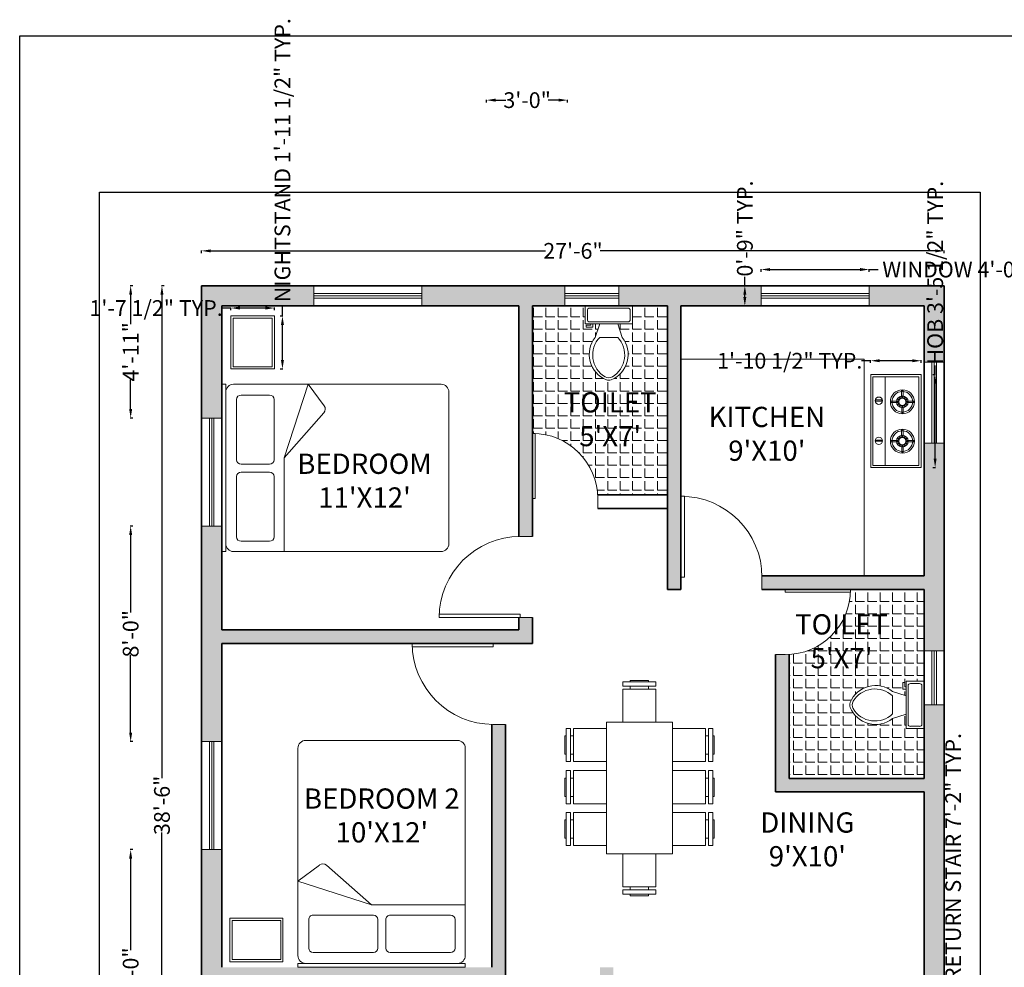
# Model space of a CAD drawing. Units: inches. Extents: x -80 to 1461, y -1239 to 153.
# Tile 3 of 6: x -80 to 358, y -273 to 149. Entities that reach past the tile are written whole.
import ezdxf

# ---------------------------------------------------------------- set-up
doc = ezdxf.new("R2010")
doc.units = ezdxf.units.IN
doc.header["$MEASUREMENT"] = 0
for name, color, linetype, lineweight in [('A-ANNO-DIMS', 2, 'Continuous', 18), ('A-ANNO-TTLB', 7, 'Continuous', 25), ('A-AREA-IDEN', 7, 'Continuous', 18), ('A-EQPM', 8, 'Continuous', 18), ('A-FLOR-FIXT', 9, 'Continuous', 18), ('A-FLOR-PATT', 143, 'Continuous', 13), ('A-FURN', 8, 'Continuous', 18), ('A-GLAZ', 4, 'Continuous', 18), ('A-WALL', 7, 'Continuous', 35), ('A-WALL-PATT', 8, 'Continuous', 13), ('DOOR', 32, 'Continuous', 18)]:
    doc.layers.add(name, color=color, linetype=linetype, lineweight=lineweight)
doc.styles.get("Standard").update_dxf_attribs({"font": 'arial.ttf'})
doc.dimstyles.get("Standard").update_dxf_attribs({"dimtxt": 7, "dimasz": 4, "dimexe": 0.18, "dimexo": 0.0625, "dimgap": 0.09, "dimtad": 0, "dimdec": 0, "dimzin": 0, "dimdsep": 46, "dimlunit": 3, "dimtxsty": 'Standard', "dimcen": 0.09, "dimadec": 0, "dimazin": 0, "dimtfac": 1, "dimtdec": 0, "dimtofl": 0, "dimtmove": 0, "dimatfit": 3, "dimfxl": 1, "dimfxlon": 1, "dimtolj": 1, "dimtzin": 0, "dimarcsym": 0})

# ---------------------------------------------------------------- blocks, each defined once
blk = doc.blocks.new('*U2')
for p, q in [((0, 0), (0, -6)), ((40, 0), (40, -6))]:
    blk.add_line(p, q)
blk.add_lwpolyline([(0, 0), (0, 40), (1.75, 40), (1.75, 0)], close=True)
blk.add_arc((0, 0), 40, 0, 90)
blk = doc.blocks.new('A$C164346CA')
for p, q in [((0, 2.035), (0, 2)), ((1.5, 2.035), (0, 2.035)), ((1.5, 2), (1.5, 2.035)), ((1.5, 2), (0, 2)), ((0, 1.93), (0, 0.07)), ((0.0919, 1.8624), (0.0919, 1.6069)), ((0.6731, 1.9024), (0.1319, 1.9024)), ((0.7131, 1.6069), (0.7131, 1.8624)), ((0.7828, 1.8624), (0.7828, 1.6069)), ((1.364, 1.9024), (0.8228, 1.9024)), ((1.404, 1.6069), (1.404, 1.8624)), ((1.5, 0.07), (1.5, 1.93)), ((0.1319, 1.5669), (0.6731, 1.5669)), ((0.8228, 1.5669), (1.364, 1.5669)), ((0.8395, 1.4761), (0, 1.4761)), ((0.8395, 1.4761), (1.2448, 1.12)), ((1.5, 1.2611), (0.8395, 1.4761)), ((1.3077, 1.1175), (1.5, 1.2611)), ((0.07, 0), (1.43, 0))]:
    blk.add_line(p, q)
for centre, radius, start, end in [((0.07, 1.93), 0.07, 90, 180), ((1.43, 1.93), 0.07, 0, 90), ((0.1319, 1.8624), 0.04, 90, 180), ((0.6731, 1.8624), 0.04, 0, 90), ((0.8228, 1.8624), 0.04, 90, 180), ((1.364, 1.8624), 0.04, 0, 90), ((0.1319, 1.6069), 0.04, 180, 270), ((0.6731, 1.6069), 0.04, 270, 0), ((0.8228, 1.6069), 0.04, 180, 270), ((1.364, 1.6069), 0.04, 270, 0), ((1.2778, 1.1575), 0.05, 228.69584, 306.75789), ((0.07, 0.07), 0.07, 180, 270), ((1.43, 0.07), 0.07, 270, 0)]:
    blk.add_arc(centre, radius, start, end)
blk = doc.blocks.new('*U5')
for p, q in [((241, -152), (241, -51)), ((-254, -216), (-203, -216)), ((-254, -241), (-254, -216)), ((-203, -216), (-203, -203)), ((-178, -203), (-178, -241)), ((-102, -203), (-152, -356)), ((102, -203), (152, -356)), ((-178, -241), (-254, -241)), ((102, -356), (-102, -356))]:
    blk.add_line(p, q)
blk.add_lwpolyline([(267, -203), (267, 0), (-267, 0), (-267, -203)], close=True)
for points in [[(-241, -51), (-241, -152)], [(216, -25), (-216, -25)], [(-216, -178), (216, -178)]]:
    blk.add_lwpolyline(points)
for centre, radius, start, end in [((-219, -48), 22.5, 81.8699, 188.1301), ((219, -48), 22.5, 351.8699, 98.1301), ((-219, -156), 22.5, 171.8699, 278.1301), ((219, -156), 22.5, 261.8699, 8.1301), ((89, -548), 309, 141.4691, 247.9714), ((107, -554), 288, 136.3677, 238.9468), ((-89, -548), 309, 292.0284, 38.5307), ((-107, -554), 288, 301.053, 43.6321), ((0, -708), 102, 245.7318, 294.2682), ((0, -737), 102, 254.8605, 285.1395)]:
    blk.add_arc(centre, radius, start, end)
blk = doc.blocks.new('A$C06E242FC')
for p, q in [((0, 455.6), (0.5, 456.1)), ((0, 455.6), (0, 0.5)), ((838.9, 456.1), (0.5, 456.1)), ((838.9, 456.1), (839.4, 455.6)), ((839.4, 0.5), (839.4, 455.6)), ((20, 435.6), (20.5, 436.1)), ((20, 435.6), (20, 20.5)), ((818.9, 436.1), (20.5, 436.1)), ((237.3, 411.5), (237.3, 356.2)), ((248.9, 411.5), (237.3, 411.5)), ((237.3, 356.2), (248.9, 356.2)), ((248.9, 356.2), (248.9, 411.5)), ((599.3, 411.5), (610.9, 411.5)), ((599.3, 411.5), (599.3, 356.2)), ((599.3, 356.2), (610.9, 356.2)), ((610.9, 356.2), (610.9, 411.5)), ((819.4, 435.6), (818.9, 436.1)), ((819.4, 20.5), (819.4, 435.6)), ((20, 324.4), (819.4, 324.4)), ((232.7, 272.7), (232.7, 214)), ((244.9, 272.7), (232.7, 272.7)), ((244.9, 214), (244.9, 272.7)), ((588.1, 272.7), (588.1, 214)), ((600.3, 272.7), (588.1, 272.7)), ((600.3, 214), (600.3, 272.7)), ((232.7, 214), (244.9, 214)), ((588.1, 214), (600.3, 214)), ((136.3, 176), (136.3, 163.8)), ((194.9, 176), (136.3, 176)), ((136.3, 163.8), (194.9, 163.8)), ((194.9, 163.8), (194.9, 176)), ((245.2, 126.1), (233, 126.1)), ((233, 126.1), (233, 67.4)), ((245.2, 67.4), (245.2, 126.1)), ((282.9, 176.3), (282.9, 164.1)), ((341.6, 176.3), (282.9, 176.3)), ((282.9, 164.1), (341.6, 164.1)), ((341.6, 164.1), (341.6, 176.3)), ((550.3, 176), (491.7, 176)), ((491.7, 176), (491.7, 163.8)), ((491.7, 163.8), (550.3, 163.8)), ((550.3, 163.8), (550.3, 176)), ((600.6, 126.1), (588.3, 126.1)), ((588.3, 126.1), (588.3, 67.4)), ((600.6, 67.4), (600.6, 126.1)), ((638.3, 176.3), (638.3, 164.1)), ((697, 176.3), (638.3, 176.3)), ((638.3, 164.1), (697, 164.1)), ((697, 164.1), (697, 176.3)), ((0, 0.5), (0.5, 0)), ((20, 20.5), (20.5, 20)), ((20.5, 20), (818.9, 20)), ((233, 67.4), (245.2, 67.4)), ((588.3, 67.4), (600.6, 67.4)), ((818.9, 20), (819.4, 20.5)), ((838.9, 0), (839.4, 0.5)), ((0.5, 0), (838.9, 0))]:
    blk.add_line(p, q)
for centre, radius in [((242, 382.9), 33.3), ((604.1, 382.9), 33.3), ((238.9, 170.1), 108.3), ((594.3, 170.1), 108.3), ((238.9, 170.1), 93.3), ((238.9, 170.1), 52.6), ((205.3, 189.5), 4.84), ((238.9, 170.1), 32.6), ((219.5, 203.7), 4.84), ((238.9, 208.9), 4.84), ((258.4, 203.7), 4.84), ((272.6, 189.5), 4.84), ((594.3, 170.1), 93.3), ((594.3, 170.1), 52.6), ((560.7, 189.5), 4.84), ((594.3, 170.1), 32.6), ((574.9, 203.7), 4.84), ((594.3, 208.9), 4.84), ((613.7, 203.7), 4.84), ((628, 189.5), 4.84), ((200.1, 170.1), 4.84), ((205.3, 150.6), 4.84), ((219.5, 136.4), 4.84), ((238.9, 131.2), 4.84), ((258.4, 136.4), 4.84), ((272.6, 150.6), 4.84), ((277.8, 170.1), 4.84), ((555.5, 170.1), 4.84), ((560.7, 150.6), 4.84), ((574.9, 136.4), 4.84), ((594.3, 131.2), 4.84), ((613.7, 136.4), 4.84), ((628, 150.6), 4.84), ((633.2, 170.1), 4.84)]:
    blk.add_circle(centre, radius)
blk = doc.blocks.new('A$C4C0603CD')
for p, q in [((1.106, 2.02), (0.656, 2.02)), ((0.656, 2.02), (0.656, 1.96)), ((1.006, 2.04), (0.756, 2.04)), ((0.756, 2.04), (0.756, 2.02)), ((1.006, 2.02), (1.006, 2.04)), ((1.106, 1.96), (1.106, 2.02)), ((1.232, 2.02), (1.232, 1.96)), ((1.684, 2.02), (1.232, 2.02)), ((1.584, 2.04), (1.334, 2.04)), ((1.334, 2.04), (1.334, 2.02)), ((1.584, 2.02), (1.584, 2.04)), ((1.684, 1.96), (1.684, 2.02)), ((1.802, 2.02), (1.802, 1.96)), ((2.252, 2.02), (1.802, 2.02)), ((2.152, 2.04), (1.902, 2.04)), ((1.902, 2.04), (1.902, 2.02)), ((2.152, 2.02), (2.152, 2.04)), ((2.252, 1.96), (2.252, 2.02)), ((1.106, 1.96), (0.656, 1.96)), ((0.656, 1.92), (0.656, 1.47)), ((1.106, 1.92), (0.656, 1.92)), ((0.756, 1.96), (0.756, 1.92)), ((1.006, 1.92), (1.006, 1.96)), ((1.106, 1.47), (1.106, 1.92)), ((1.684, 1.96), (1.232, 1.96)), ((1.232, 1.92), (1.232, 1.47)), ((1.684, 1.92), (1.232, 1.92)), ((1.334, 1.96), (1.334, 1.92)), ((1.584, 1.92), (1.584, 1.96)), ((1.684, 1.47), (1.684, 1.92)), ((2.252, 1.96), (1.802, 1.96)), ((1.802, 1.92), (1.802, 1.47)), ((2.252, 1.92), (1.802, 1.92)), ((1.902, 1.96), (1.902, 1.92)), ((2.152, 1.92), (2.152, 1.96)), ((2.252, 1.47), (2.252, 1.92)), ((0.57, 1.47), (0.57, 0.57)), ((2.37, 1.47), (0.57, 1.47)), ((0.656, 1.47), (1.106, 1.47)), ((1.107, 1.47), (1.684, 1.47)), ((1.802, 1.47), (2.252, 1.47)), ((2.37, 1.47), (2.37, 0.57)), ((0.02, 1.245), (0.02, 0.795)), ((0.08, 1.245), (0.02, 1.245)), ((0.08, 1.245), (0.08, 0.795)), ((0.12, 1.245), (0.12, 0.795)), ((0.57, 1.245), (0.12, 1.245)), ((0.57, 0.795), (0.57, 1.245)), ((2.37, 1.245), (2.37, 0.795)), ((2.82, 1.245), (2.37, 1.245)), ((2.82, 0.795), (2.82, 1.245)), ((2.86, 0.795), (2.86, 1.245)), ((2.92, 1.245), (2.86, 1.245)), ((2.92, 0.795), (2.92, 1.245)), ((0, 1.145), (0, 0.895)), ((0.02, 1.145), (0, 1.145)), ((0.12, 1.145), (0.08, 1.145)), ((2.86, 1.145), (2.82, 1.145)), ((2.94, 1.145), (2.92, 1.145)), ((2.94, 0.895), (2.94, 1.145)), ((0, 0.895), (0.02, 0.895)), ((0.08, 0.895), (0.12, 0.895)), ((2.82, 0.895), (2.86, 0.895)), ((2.92, 0.895), (2.94, 0.895)), ((0.02, 0.795), (0.08, 0.795)), ((0.12, 0.795), (0.57, 0.795)), ((2.37, 0.795), (2.82, 0.795)), ((2.86, 0.795), (2.92, 0.795)), ((0.57, 0.57), (2.37, 0.57)), ((1.106, 0.57), (0.656, 0.57)), ((0.656, 0.57), (0.656, 0.12)), ((1.106, 0.12), (1.106, 0.57)), ((1.684, 0.57), (1.232, 0.57)), ((1.232, 0.57), (1.232, 0.12)), ((1.684, 0.12), (1.684, 0.57)), ((2.252, 0.57), (1.802, 0.57)), ((1.802, 0.57), (1.802, 0.12)), ((2.252, 0.12), (2.252, 0.57)), ((0.656, 0.12), (1.106, 0.12)), ((0.656, 0.08), (1.106, 0.08)), ((0.656, 0.08), (0.656, 0.02)), ((0.656, 0.02), (1.106, 0.02)), ((0.756, 0.12), (0.756, 0.08)), ((0.756, 0.02), (0.756, 0)), ((0.756, 0), (1.006, 0)), ((1.006, 0.08), (1.006, 0.12)), ((1.006, 0), (1.006, 0.02)), ((1.106, 0.02), (1.106, 0.08)), ((1.232, 0.12), (1.684, 0.12)), ((1.232, 0.08), (1.684, 0.08)), ((1.232, 0.08), (1.232, 0.02)), ((1.232, 0.02), (1.684, 0.02)), ((1.334, 0.12), (1.334, 0.08)), ((1.334, 0.02), (1.334, 0)), ((1.334, 0), (1.584, 0)), ((1.584, 0.08), (1.584, 0.12)), ((1.584, 0), (1.584, 0.02)), ((1.684, 0.02), (1.684, 0.08)), ((1.802, 0.12), (2.252, 0.12)), ((1.802, 0.08), (2.252, 0.08)), ((1.802, 0.08), (1.802, 0.02)), ((1.802, 0.02), (2.252, 0.02)), ((1.902, 0.12), (1.902, 0.08)), ((1.902, 0.02), (1.902, 0)), ((1.902, 0), (2.152, 0)), ((2.152, 0.08), (2.152, 0.12)), ((2.152, 0), (2.152, 0.02)), ((2.252, 0.02), (2.252, 0.08))]:
    blk.add_line(p, q)
blk = doc.blocks.new('*D11')
at = {"layer": 'A-ANNO-DIMS', "color": 0, "lineweight": -2, "transparency": 16777216}
for p, q in [((0.99, 44.81), (0.99, 45.99)), ((4.99, 45.81), (153.82, 45.81)), ((326.99, 45.81), (178.16, 45.81)), ((330.99, 44.81), (330.99, 45.99))]:
    blk.add_line(p, q, dxfattribs=at)
at = {"layer": 'A-ANNO-DIMS', "color": 0, "transparency": 16777216}
for points in [[(4.99, 46.47), (4.99, 45.14), (0.99, 45.81)], [(326.99, 46.47), (326.99, 45.14), (330.99, 45.81)]]:
    blk.add_solid(points, dxfattribs=at)
at = {"layer": 'Defpoints', "color": 0, "transparency": 16777216}
for p in [(330.99, 45.81), (0.99, 30.32), (330.99, 30.32)]:
    blk.add_point(p, dxfattribs=at)
at = {"layer": 'A-ANNO-DIMS', "color": 0, "transparency": 16777216, "insert": (165.99, 45.81), "char_height": 7, "attachment_point": 5}
blk.add_mtext('\\A1;27\'-6"', dxfattribs=at)
blk = doc.blocks.new('*D12')
at = {"layer": 'A-ANNO-DIMS', "color": 0, "lineweight": -2, "transparency": 16777216}
for p, q in [((-15.61, 30.32), (-16.79, 30.32)), ((-16.61, 26.32), (-16.61, -188.57)), ((-16.61, -427.68), (-16.61, -212.8)), ((-15.61, -431.68), (-16.79, -431.68))]:
    blk.add_line(p, q, dxfattribs=at)
at = {"layer": 'A-ANNO-DIMS', "color": 0, "transparency": 16777216}
for points in [[(-17.27, 26.32), (-15.94, 26.32), (-16.61, 30.32)], [(-17.27, -427.68), (-15.94, -427.68), (-16.61, -431.68)]]:
    blk.add_solid(points, dxfattribs=at)
at = {"layer": 'Defpoints', "color": 0, "transparency": 16777216}
for p in [(0.99, 30.32), (-16.61, -431.68), (0.99, -431.68)]:
    blk.add_point(p, dxfattribs=at)
at = {"layer": 'A-ANNO-DIMS', "color": 0, "transparency": 16777216, "insert": (-16.61, -200.68), "char_height": 7, "attachment_point": 5, "rotation": 90}
blk.add_mtext('\\A1;38\'-6"', dxfattribs=at)
blk = doc.blocks.new('WIN-48IN')
for p, q in [((0, 9), (0, 0)), ((48, 9), (0, 9)), ((48, 0), (48, 9)), ((0, 5.5), (48, 5.5)), ((0, 4.5), (48, 4.5)), ((0, 3.5), (48, 3.5)), ((0, 0), (36, 0)), ((36, 0), (48, 0))]:
    blk.add_line(p, q)
blk = doc.blocks.new('WIN-24IN')
for p, q in [((0, 9), (0, 0)), ((0, 9), (24, 9)), ((24, 9), (24, 0)), ((0, 5.5), (24, 5.5)), ((0, 4.5), (24, 4.5)), ((0, 3.5), (24, 3.5)), ((0, 0), (24, 0))]:
    blk.add_line(p, q)
blk = doc.blocks.new('WIN-36IN')
for p, q in [((0, 36), (9, 36)), ((0, 36), (0, 0)), ((3.5, 0), (3.5, 36)), ((4.5, 0), (4.5, 36)), ((5.5, 0), (5.5, 36)), ((9, 0), (9, 36)), ((0, 0), (9, 0))]:
    blk.add_line(p, q)
blk = doc.blocks.new('NIGHTSTAND')
for points in [[(0, 19.36), (23.56, 19.36), (23.56, 0), (0, 0)], [(1, 18.36), (22.56, 18.36), (22.56, 1), (1, 1)]]:
    blk.add_lwpolyline(points, close=True)
blk = doc.blocks.new('COUNTER-L-PLAN')
for p, q in [((0, 96.29), (81.45, 96.29)), ((81.45, 96.29), (81.45, 0))]:
    blk.add_line(p, q)
blk = doc.blocks.new('*D36')
at = {"layer": 'A-ANNO-DIMS', "color": 0, "lineweight": -2, "transparency": 16777216}
for p, q in [((249.57, 36.52), (249.57, 37.7)), ((253.57, 37.52), (293.57, 37.52)), ((297.57, 36.52), (297.57, 37.7)), ((297.57, 37.52), (301.57, 37.52))]:
    blk.add_line(p, q, dxfattribs=at)
at = {"layer": 'A-ANNO-DIMS', "color": 0, "transparency": 16777216}
for points in [[(253.57, 38.18), (253.57, 36.85), (249.57, 37.52)], [(293.57, 38.18), (293.57, 36.85), (297.57, 37.52)]]:
    blk.add_solid(points, dxfattribs=at)
at = {"layer": 'Defpoints', "color": 0, "transparency": 16777216}
for p in [(297.57, 37.52), (249.57, 30.32), (297.57, 30.32)]:
    blk.add_point(p, dxfattribs=at)
at = {"layer": 'A-ANNO-DIMS', "color": 0, "transparency": 16777216, "insert": (345.95, 37.52), "char_height": 7, "attachment_point": 5}
blk.add_mtext('\\A1;WINDOW 4\'-0" TYP.', dxfattribs=at)
blk = doc.blocks.new('*D37')
at = {"layer": 'A-ANNO-DIMS', "color": 0, "lineweight": -2, "transparency": 16777216}
for p, q in [((242.37, 30.32), (242.37, 34.32)), ((243.37, 30.32), (242.19, 30.32)), ((242.37, 25.32), (242.37, 26.32)), ((243.37, 21.32), (242.19, 21.32))]:
    blk.add_line(p, q, dxfattribs=at)
at = {"layer": 'A-ANNO-DIMS', "color": 0, "transparency": 16777216}
for points in [[(241.7, 26.32), (243.03, 26.32), (242.37, 30.32)], [(241.7, 25.32), (243.03, 25.32), (242.37, 21.32)]]:
    blk.add_solid(points, dxfattribs=at)
at = {"layer": 'Defpoints', "color": 0, "transparency": 16777216}
for p in [(242.37, 30.32), (249.57, 30.32), (249.57, 21.32)]:
    blk.add_point(p, dxfattribs=at)
at = {"layer": 'A-ANNO-DIMS', "color": 0, "transparency": 16777216, "insert": (242.37, 55.74), "char_height": 7, "attachment_point": 5, "rotation": 90}
blk.add_mtext('\\A1;0\'-9" TYP.', dxfattribs=at)
blk = doc.blocks.new('*D48')
at = {"layer": 'A-ANNO-DIMS', "color": 0, "lineweight": -2, "transparency": 16777216}
for p, q in [((36.92, 16.87), (36.92, 20.87)), ((35.92, 16.87), (37.1, 16.87)), ((36.92, -2.69), (36.92, 12.87)), ((35.92, -6.69), (37.1, -6.69))]:
    blk.add_line(p, q, dxfattribs=at)
at = {"layer": 'A-ANNO-DIMS', "color": 0, "transparency": 16777216}
for points in [[(36.25, 12.87), (37.59, 12.87), (36.92, 16.87)], [(36.25, -2.69), (37.59, -2.69), (36.92, -6.69)]]:
    blk.add_solid(points, dxfattribs=at)
at = {"layer": 'Defpoints', "color": 0, "transparency": 16777216}
for p in [(33.39, 16.87), (36.92, 16.87), (33.39, -6.69)]:
    blk.add_point(p, dxfattribs=at)
at = {"layer": 'A-ANNO-DIMS', "color": 0, "transparency": 16777216, "insert": (36.92, 86.13), "char_height": 7, "attachment_point": 5, "rotation": 90}
blk.add_mtext('\\A1;NIGHTSTAND 1\'-11 1/2" TYP.', dxfattribs=at)
blk = doc.blocks.new('*D49')
at = {"layer": 'A-ANNO-DIMS', "color": 0, "lineweight": -2, "transparency": 16777216}
for p, q in [((14.03, 20.4), (10.03, 20.4)), ((14.03, 19.4), (14.03, 20.58)), ((29.39, 20.4), (18.03, 20.4)), ((33.39, 19.4), (33.39, 20.58))]:
    blk.add_line(p, q, dxfattribs=at)
at = {"layer": 'A-ANNO-DIMS', "color": 0, "transparency": 16777216}
for points in [[(18.03, 21.07), (18.03, 19.73), (14.03, 20.4)], [(29.39, 21.07), (29.39, 19.73), (33.39, 20.4)]]:
    blk.add_solid(points, dxfattribs=at)
at = {"layer": 'Defpoints', "color": 0, "transparency": 16777216}
for p in [(14.03, 20.4), (14.03, 16.87), (33.39, 16.87)]:
    blk.add_point(p, dxfattribs=at)
at = {"layer": 'A-ANNO-DIMS', "color": 0, "transparency": 16777216, "insert": (-19.22, 20.4), "char_height": 7, "attachment_point": 5}
blk.add_mtext('\\A1;1\'-7 1/2" TYP.', dxfattribs=at)
blk = doc.blocks.new('*D50')
at = {"layer": 'A-ANNO-DIMS', "color": 0, "lineweight": -2, "transparency": 16777216}
for p, q in [((326.92, -9.22), (326.92, -5.22)), ((325.92, -9.22), (327.1, -9.22)), ((326.92, -46.53), (326.92, -13.22)), ((325.92, -50.53), (327.1, -50.53))]:
    blk.add_line(p, q, dxfattribs=at)
at = {"layer": 'A-ANNO-DIMS', "color": 0, "transparency": 16777216}
for points in [[(326.25, -13.22), (327.58, -13.22), (326.92, -9.22)], [(326.25, -46.53), (327.58, -46.53), (326.92, -50.53)]]:
    blk.add_solid(points, dxfattribs=at)
at = {"layer": 'Defpoints', "color": 0, "transparency": 16777216}
for p in [(320.72, -9.22), (326.92, -9.22), (320.72, -50.53)]:
    blk.add_point(p, dxfattribs=at)
at = {"layer": 'A-ANNO-DIMS', "color": 0, "transparency": 16777216, "insert": (326.92, 36.12), "char_height": 7, "attachment_point": 5, "rotation": 90}
blk.add_mtext('\\A1;HOB 3\'-5 1/2" TYP.', dxfattribs=at)
blk = doc.blocks.new('*D51')
at = {"layer": 'A-ANNO-DIMS', "color": 0, "lineweight": -2, "transparency": 16777216}
for p, q in [((298.27, -3.03), (294.27, -3.03)), ((298.27, -4.03), (298.27, -2.85)), ((316.72, -3.03), (302.27, -3.03)), ((320.72, -4.03), (320.72, -2.85))]:
    blk.add_line(p, q, dxfattribs=at)
at = {"layer": 'A-ANNO-DIMS', "color": 0, "transparency": 16777216}
for points in [[(302.27, -2.36), (302.27, -3.69), (298.27, -3.03)], [(316.72, -2.36), (316.72, -3.69), (320.72, -3.03)]]:
    blk.add_solid(points, dxfattribs=at)
at = {"layer": 'Defpoints', "color": 0, "transparency": 16777216}
for p in [(298.27, -3.03), (298.27, -9.22), (320.72, -9.22)]:
    blk.add_point(p, dxfattribs=at)
at = {"layer": 'A-ANNO-DIMS', "color": 0, "transparency": 16777216, "insert": (262.3, -3.03), "char_height": 7, "attachment_point": 5}
blk.add_mtext('\\A1;1\'-10 1/2" TYP.', dxfattribs=at)
blk = doc.blocks.new('*D56')
at = {"layer": 'A-ANNO-DIMS', "color": 0, "lineweight": -2, "transparency": 16777216}
for p, q in [((334.89, -286.42), (334.89, -282.42)), ((333.89, -286.42), (335.07, -286.42)), ((334.89, -368.42), (334.89, -290.42)), ((333.89, -372.42), (335.07, -372.42))]:
    blk.add_line(p, q, dxfattribs=at)
at = {"layer": 'A-ANNO-DIMS', "color": 0, "transparency": 16777216}
for points in [[(334.22, -290.42), (335.56, -290.42), (334.89, -286.42)], [(334.22, -368.42), (335.56, -368.42), (334.89, -372.42)]]:
    blk.add_solid(points, dxfattribs=at)
at = {"layer": 'Defpoints', "color": 0, "transparency": 16777216}
for p in [(321.99, -286.42), (334.89, -286.42), (321.99, -372.42)]:
    blk.add_point(p, dxfattribs=at)
at = {"layer": 'A-ANNO-DIMS', "color": 0, "transparency": 16777216, "insert": (334.89, -223.69), "char_height": 7, "attachment_point": 5, "rotation": 90}
blk.add_mtext('\\A1;RETURN STAIR 7\'-2" TYP.', dxfattribs=at)
blk = doc.blocks.new('*D72')
at = {"layer": 'A-ANNO-DIMS', "color": 0, "lineweight": -2, "transparency": 16777216}
for p, q in [((412.49, 30.32), (413.67, 30.32)), ((413.49, 26.32), (413.49, -224.38)), ((413.49, -499.58), (413.49, -248.89)), ((412.49, -503.58), (413.67, -503.58))]:
    blk.add_line(p, q, dxfattribs=at)
at = {"layer": 'A-ANNO-DIMS', "color": 0, "transparency": 16777216}
for points in [[(412.82, 26.32), (414.16, 26.32), (413.49, 30.32)], [(412.82, -499.58), (414.16, -499.58), (413.49, -503.58)]]:
    blk.add_solid(points, dxfattribs=at)
at = {"layer": 'Defpoints', "color": 0, "transparency": 16777216}
for p in [(330.99, 30.32), (183.99, -503.58), (413.49, -503.58)]:
    blk.add_point(p, dxfattribs=at)
at = {"layer": 'A-ANNO-DIMS', "color": 0, "transparency": 16777216, "insert": (413.49, -236.63), "char_height": 7, "attachment_point": 5, "rotation": 90}
blk.add_mtext('\\A1;44\'-6"', dxfattribs=at)
blk = doc.blocks.new('*D74')
at = {"layer": 'A-ANNO-DIMS', "color": 0, "lineweight": -2, "transparency": 16777216}
for p, q in [((127.63, 111.82), (127.63, 113)), ((131.63, 112.82), (136.23, 112.82)), ((159.62, 112.82), (155.02, 112.82)), ((163.62, 111.82), (163.62, 113))]:
    blk.add_line(p, q, dxfattribs=at)
at = {"layer": 'A-ANNO-DIMS', "color": 0, "transparency": 16777216}
for points in [[(131.63, 113.48), (131.63, 112.15), (127.63, 112.82)], [(159.62, 113.48), (159.62, 112.15), (163.62, 112.82)]]:
    blk.add_solid(points, dxfattribs=at)
at = {"layer": 'Defpoints', "color": 0, "transparency": 16777216}
for p in [(163.62, 112.82), (127.63, -431.68), (163.62, -431.68)]:
    blk.add_point(p, dxfattribs=at)
at = {"layer": 'A-ANNO-DIMS', "color": 0, "transparency": 16777216, "insert": (145.63, 112.82), "char_height": 7, "attachment_point": 5}
blk.add_mtext('\\A1;3\'-0"', dxfattribs=at)
blk = doc.blocks.new('*D76')
at = {"layer": 'A-ANNO-DIMS', "color": 0, "lineweight": -2, "transparency": 16777216}
for p, q in [((147.99, -534.08), (147.99, -535.26)), ((151.99, -535.08), (153.04, -535.08)), ((172.99, -535.08), (171.94, -535.08)), ((176.99, -534.08), (176.99, -535.26))]:
    blk.add_line(p, q, dxfattribs=at)
at = {"layer": 'A-ANNO-DIMS', "color": 0, "transparency": 16777216}
for points in [[(151.99, -534.42), (151.99, -535.75), (147.99, -535.08)], [(172.99, -534.42), (172.99, -535.75), (176.99, -535.08)]]:
    blk.add_solid(points, dxfattribs=at)
at = {"layer": 'Defpoints', "color": 0, "transparency": 16777216}
for p in [(147.99, -68.68), (176.99, -68.68), (176.99, -535.08)]:
    blk.add_point(p, dxfattribs=at)
at = {"layer": 'A-ANNO-DIMS', "color": 0, "transparency": 16777216, "insert": (162.49, -535.08), "char_height": 7, "attachment_point": 5}
blk.add_mtext('\\A1;2\'-5"', dxfattribs=at)
blk = doc.blocks.new('*D81')
at = {"layer": 'A-ANNO-DIMS', "color": 0, "lineweight": -2, "transparency": 16777216}
for p, q in [((-29.51, 30.32), (-30.69, 30.32)), ((-30.51, 26.32), (-30.51, 13.16)), ((-30.51, -24.5), (-30.51, -11.34)), ((-29.51, -28.5), (-30.69, -28.5))]:
    blk.add_line(p, q, dxfattribs=at)
at = {"layer": 'A-ANNO-DIMS', "color": 0, "transparency": 16777216}
for points in [[(-31.18, 26.32), (-29.84, 26.32), (-30.51, 30.32)], [(-31.18, -24.5), (-29.84, -24.5), (-30.51, -28.5)]]:
    blk.add_solid(points, dxfattribs=at)
at = {"layer": 'Defpoints', "color": 0, "transparency": 16777216}
for p in [(0.99, 30.32), (-30.51, -28.5), (0.99, -28.5)]:
    blk.add_point(p, dxfattribs=at)
at = {"layer": 'A-ANNO-DIMS', "color": 0, "transparency": 16777216, "insert": (-30.51, 0.91), "char_height": 7, "attachment_point": 5, "rotation": 90}
blk.add_mtext('\\A1;4\'-11"', dxfattribs=at)
blk = doc.blocks.new('*D82')
at = {"layer": 'A-ANNO-DIMS', "color": 0, "lineweight": -2, "transparency": 16777216}
for p, q in [((-29.51, -76.5), (-30.69, -76.5)), ((-30.51, -80.5), (-30.51, -115.02)), ((-30.51, -168.33), (-30.51, -133.81)), ((-29.51, -172.33), (-30.69, -172.33))]:
    blk.add_line(p, q, dxfattribs=at)
at = {"layer": 'A-ANNO-DIMS', "color": 0, "transparency": 16777216}
for points in [[(-31.18, -80.5), (-29.84, -80.5), (-30.51, -76.5)], [(-31.18, -168.33), (-29.84, -168.33), (-30.51, -172.33)]]:
    blk.add_solid(points, dxfattribs=at)
at = {"layer": 'Defpoints', "color": 0, "transparency": 16777216}
for p in [(0.99, -76.5), (-30.51, -172.33), (0.99, -172.33)]:
    blk.add_point(p, dxfattribs=at)
at = {"layer": 'A-ANNO-DIMS', "color": 0, "transparency": 16777216, "insert": (-30.51, -124.41), "char_height": 7, "attachment_point": 5, "rotation": 90}
blk.add_mtext('\\A1;8\'-0"', dxfattribs=at)
blk = doc.blocks.new('*D83')
at = {"layer": 'A-ANNO-DIMS', "color": 0, "lineweight": -2, "transparency": 16777216}
for p, q in [((-29.51, -220.33), (-30.69, -220.33)), ((-30.51, -224.33), (-30.51, -265)), ((-30.51, -324.45), (-30.51, -283.78)), ((-29.51, -328.45), (-30.69, -328.45))]:
    blk.add_line(p, q, dxfattribs=at)
at = {"layer": 'A-ANNO-DIMS', "color": 0, "transparency": 16777216}
for points in [[(-31.18, -224.33), (-29.84, -224.33), (-30.51, -220.33)], [(-31.18, -324.45), (-29.84, -324.45), (-30.51, -328.45)]]:
    blk.add_solid(points, dxfattribs=at)
at = {"layer": 'Defpoints', "color": 0, "transparency": 16777216}
for p in [(0.99, -220.33), (-30.51, -328.45), (0.99, -328.45)]:
    blk.add_point(p, dxfattribs=at)
at = {"layer": 'A-ANNO-DIMS', "color": 0, "transparency": 16777216, "insert": (-30.51, -274.39), "char_height": 7, "attachment_point": 5, "rotation": 90}
blk.add_mtext('\\A1;9\'-0"', dxfattribs=at)

msp = doc.modelspace()

# ---------------------------------------------------------------- hatches: boundary and pattern name
at = {"layer": 'A-FLOR-PATT'}
h = msp.add_hatch(dxfattribs=at)
h.set_pattern_fill('ANGLE', color=256, scale=20)
h.set_pattern_definition([(0, (0, 0), (0, 5.5), [4, -1.5]), (90, (0, 0), (-5.5, 3e-16), [4, -1.5])])
h.paths.add_polyline_path([(207.99, 21.32), (192.39, 21.32), (192.39, 13.32), (185.89, 13.32), (187.89, 7.32, -0.501323), (182.94, -11.55, -0.132891), (180.85, -11.55, -0.501317), (175.89, 7.32), (177.89, 13.32), (174.89, 13.32), (174.89, 11.82), (171.89, 11.82), (171.89, 12.82), (173.89, 12.82), (173.89, 13.32), (171.39, 13.32), (171.39, 21.32), (162.37, 21.32), (147.99, 21.32), (147.99, -35.33), (149.26, -35.33), (149.26, -35.36, -0.38502), (176.94, -62.68), (207.99, -62.68)])
h.paths.add_polyline_path([(321.99, -104.68), (289.34, -104.68), (289.34, -105.95), (289.31, -105.95, -0.38502), (261.99, -133.64), (261.99, -188.68), (321.99, -188.68), (321.99, -166.56), (313.99, -166.56), (313.99, -160.06), (307.99, -162.06, -0.501323), (289.13, -157.1, -0.132891), (289.13, -155.01, -0.501317), (307.99, -150.06), (313.99, -152.06), (313.99, -149.06), (312.49, -149.06), (312.49, -146.06), (313.99, -146.06), (313.99, -145.56), (321.99, -145.56)])
at = {"layer": 'A-WALL-PATT'}
h = msp.add_hatch(color=256, dxfattribs=at)
h.dxf.hatch_style = 1
h.paths.add_polyline_path([(9.99, -76.5), (0.99, -76.5), (0.99, -172.33), (9.99, -172.33), (9.99, -128.68), (147.99, -128.68), (147.99, -117.2), (142.59, -117.2), (141.99, -117.2), (141.99, -122.68), (9.99, -122.68)])
h.paths.add_polyline_path([(50.86, 30.32), (0.99, 30.32), (0.99, -28.5), (9.99, -28.5), (9.99, -13.51), (9.99, 21.32), (50.86, 21.32)])
h = msp.add_hatch(color=256, dxfattribs=at)
h.dxf.hatch_style = 1
h.paths.add_polyline_path([(162.37, 30.32), (98.86, 30.32), (98.86, 21.32), (141.99, 21.32), (141.99, -81.2, -0.004167), (142.59, -81.2), (147.99, -81.2), (147.99, 21.32), (162.37, 21.32)])
h.paths.add_polyline_path([(330.99, 30.32), (297.57, 30.32), (297.57, 21.32), (321.99, 21.32), (321.99, -3.69), (330.99, -3.69)])
h.paths.add_polyline_path([(249.57, 30.32), (186.37, 30.32), (186.37, 21.32), (192.39, 21.32), (207.99, 21.32), (207.99, -104.68), (213.99, -104.68), (213.99, -99.28), (213.99, -63.28), (213.99, 21.32), (249.57, 21.32)])
h.paths.add_polyline_path([(330.99, -39.69), (321.99, -39.69), (321.99, -98.68), (249.99, -98.68, -0.004167), (249.99, -99.28), (249.99, -104.68), (321.99, -104.68), (321.99, -132.06), (330.99, -132.06)])
h.paths.add_polyline_path([(330.99, -156.06), (321.99, -156.06), (321.99, -166.56), (321.99, -188.68), (261.99, -188.68), (261.99, -133.64, -0.014233), (260.34, -133.68), (255.99, -133.68), (255.99, -194.68), (321.99, -194.68), (321.99, -372.42), (306.16, -372.42), (306.16, -381.42), (330.99, -381.42)])
h = msp.add_hatch(color=256, dxfattribs=at)
h.dxf.hatch_style = 1
h.paths.add_polyline_path([(183.99, -272.68), (177.99, -272.68), (177.99, -422.68), (163.62, -422.68), (163.62, -426.28), (163.62, -431.68), (183.99, -431.68)])
h.paths.add_polyline_path([(9.99, -220.33), (0.99, -220.33), (0.99, -328.45), (9.99, -328.45), (9.99, -278.68), (135.99, -278.68), (135.99, -272.68), (9.99, -272.68)])
h.paths.add_polyline_path([(135.99, -164.68), (130.59, -164.68, -0.004167), (129.99, -164.68), (129.99, -272.68), (135.99, -272.68)])
h.paths.add_polyline_path([(127.62, -426.28, -0.025047), (127.8, -422.68), (73.28, -422.68), (73.28, -431.68), (127.62, -431.68)])
h.paths.add_polyline_path([(25.28, -422.68), (9.99, -422.68), (9.99, -376.45), (0.99, -376.45), (0.99, -431.68), (25.28, -431.68)])

# ---------------------------------------------------------------- linework, layer by layer
at = {"layer": 'A-ANNO-TTLB'}
for points in [[(-79.81, 141.36), (1461.09, 141.36), (1461.09, -1239.28), (-79.81, -1239.28)], [(-44.36, 71.88), (346.97, 71.88), (346.97, -556.04), (-44.36, -556.04)]]:
    msp.add_lwpolyline(points, close=True, dxfattribs=at)
at = {"layer": 'A-WALL'}
for p, q in [((0.99, 30.32), (330.99, 30.32)), ((0.99, 30.32), (0.99, -431.68)), ((330.99, 30.32), (330.99, -381.42)), ((9.99, 21.32), (141.99, 21.32)), ((9.99, 21.32), (9.99, -122.68)), ((141.99, 21.32), (141.99, -81.2)), ((147.99, 21.32), (147.99, -81.2)), ((147.99, 21.32), (207.99, 21.32)), ((207.99, 21.32), (207.99, -104.68)), ((213.99, 21.32), (213.99, -104.68)), ((213.99, 21.32), (321.99, 21.32)), ((321.99, 21.32), (321.99, -98.68)), ((176.94, -62.68), (207.99, -62.68)), ((176.99, -68.68), (207.99, -68.68)), ((249.99, -98.68), (321.99, -98.68)), ((207.99, -104.68), (213.99, -104.68)), ((249.99, -104.68), (321.99, -104.68)), ((321.99, -104.68), (321.99, -188.68)), ((141.99, -117.2), (141.99, -122.68)), ((147.99, -117.2), (147.99, -128.68)), ((9.99, -122.68), (141.99, -122.68)), ((9.99, -128.68), (147.99, -128.68)), ((9.99, -128.68), (9.99, -272.68)), ((255.99, -133.68), (255.99, -194.68)), ((261.99, -133.64), (261.99, -188.68)), ((129.99, -164.68), (129.99, -272.68)), ((135.99, -164.68), (135.99, -278.68)), ((261.99, -188.68), (321.99, -188.68)), ((255.99, -194.68), (321.99, -194.68)), ((321.99, -194.68), (321.99, -372.42))]:
    msp.add_line(p, q, dxfattribs=at)

# ---------------------------------------------------------------- block references
at = {"layer": 'A-EQPM', "xscale": 0.0492111581744576, "yscale": 0.0492111581744576, "zscale": 0.0492111581744576, "rotation": 90}
msp.add_blockref('A$C06E242FC', (320.72, -50.53), dxfattribs=at)
at = {"layer": 'A-FLOR-FIXT', "xscale": 0.0393700787401575, "yscale": 0.0393700787401575, "zscale": 0.0393700787401575}
msp.add_blockref('*U5', (181.89, 21.32), dxfattribs=at)
at = {"layer": 'A-FLOR-FIXT'}
msp.add_blockref('COUNTER-L-PLAN', (213.99, -98.68), dxfattribs=at)
at = {"layer": 'A-FLOR-FIXT', "xscale": 0.0393700787401575, "yscale": 0.0393700787401575, "zscale": 0.0393700787401575, "rotation": 270}
msp.add_blockref('*U5', (321.99, -156.06), dxfattribs=at)
at = {"layer": 'A-FURN', "rotation": 90.00000000000018}
msp.add_blockref('NIGHTSTAND', (33.39, -6.69), dxfattribs=at)
at = {"layer": 'A-FURN'}
for name, p, xscale, yscale, zscale, rotation in [('A$C164346CA', (110.86, -87.86), 49.56739756478314, 49.56739756478314, 49.56739756478314, 90), ('A$C4C0603CD', (162.33, -145.12), 32.56630135070871, 32.56630135070871, 32.56630135070871, 270), ('A$C164346CA', (118.17, -171.81), 49.56739756478314, 49.56739756478314, 49.56739756478314, 180)]:
    msp.add_blockref(name, p, dxfattribs=dict(at, xscale=xscale, yscale=yscale, zscale=zscale, rotation=rotation))
msp.add_blockref('NIGHTSTAND', (13.59, -270.21), dxfattribs=at)
at = {"layer": 'A-GLAZ'}
for name, p in [('WIN-48IN', (50.86, 21.32)), ('WIN-24IN', (162.37, 21.32)), ('WIN-48IN', (249.57, 21.32)), ('WIN-36IN', (321.99, -39.69))]:
    msp.add_blockref(name, p, dxfattribs=at)
for name, p, rotation in [('WIN-48IN', (9.99, -76.5), 90.00000000000003), ('WIN-24IN', (321.99, -132.06), 269.9999999999994), ('WIN-48IN', (9.99, -220.33), 90.00000000000003)]:
    msp.add_blockref(name, p, dxfattribs=dict(at, rotation=rotation))
at = {"layer": 'DOOR'}
for p, xscale, yscale, zscale in [((147.99, -64.33), 0.7250000000000001, 0.7250000000000001, 0.7250000000000001), ((213.99, -99.28), 0.9, 0.9, 0.9)]:
    msp.add_blockref('*U2', p, dxfattribs=dict(at, xscale=xscale, yscale=yscale, zscale=zscale))
for p, xscale, yscale, zscale, rotation in [((142.59, -117.2), 0.9, 0.9, 0.9, 90), ((260.34, -104.68), 0.7250000000000001, 0.7250000000000001, 0.7250000000000001, 270), ((130.59, -128.68), -0.9, 0.9, 0.9, 90)]:
    msp.add_blockref('*U2', p, dxfattribs=dict(at, xscale=xscale, yscale=yscale, zscale=zscale, rotation=rotation))

# ---------------------------------------------------------------- texts
at = {"layer": 'A-AREA-IDEN', "char_height": 9, "attachment_point": 1}
for s, width, insert in [("\\pxqc;TOILET\\P5'X7'", 57.3791, (153.84, -17.02)), ("\\pxqc;KITCHEN\\P9'X10'", 96.7224, (203.79, -23.52)), ("\\pxqc;BEDROOM\\P11'X12'", 96.7224, (25.02, -44.33)), ("\\pxqc;TOILET\\P5'X7'", 57.3791, (256.63, -115.73)), ("\\pxqc;BEDROOM 2\\P10'X12'", 96.7224, (32.75, -193.17)), ("\\pxqc;DINING\\P9'X10'", 57.3791, (241.46, -203.81))]:
    msp.add_mtext_dynamic_manual_height_columns(s, width=width, gutter_width=1, heights=[0], dxfattribs=dict(at, insert=insert))

# ---------------------------------------------------------------- dimensions: what is measured, and where the dimension line sits
at = {"layer": 'A-ANNO-DIMS'}
for base, p1, p2, angle, text, picture, middle in [((36.92, 16.87), (33.39, -6.69), (33.39, 16.87), 90, 'NIGHTSTAND <> TYP.', '*D48', (36.92, 86.13)), ((242.37, 30.32), (249.57, 21.32), (249.57, 30.32), 90, '<> TYP.', '*D37', (242.37, 55.74)), ((326.92, -9.22), (320.72, -50.53), (320.72, -9.22), 90, 'HOB <> TYP.', '*D50', (326.92, 36.12)), ((14.03, 20.4), (33.39, 16.87), (14.03, 16.87), 180, '<> TYP.', '*D49', (-19.22, 20.4)), ((298.2742, -3.0282), (320.72, -9.2243), (298.2742, -9.2243), 180, '<> TYP.', '*D51', (262.3046, -3.0282)), ((334.89, -286.42), (321.99, -372.42), (321.99, -286.42), 90, 'RETURN STAIR <> TYP.', '*D56', (334.89, -223.69))]:
    dim = msp.add_linear_dim(base=base, p1=p1, p2=p2, angle=angle, text=text, dimstyle='Standard', override={"dimdec": 1, "dimlfac": 1, "dimrnd": 0, "dimzin": 1, "dimdsep": 46, "dimlunit": 4, "dimfrac": 2}, dxfattribs=at)
    dim.commit()
    dim.dimension.update_dxf_attribs({"geometry": picture, "text_midpoint": middle})
for base, p1, p2, override, picture, middle in [((163.62, 112.82), (127.63, -431.68), (163.62, -431.68), {"dimdec": 1, "dimlfac": 1, "dimrnd": 0, "dimzin": 1, "dimdsep": 46, "dimlunit": 4, "dimfrac": 2}, '*D74', (145.63, 112.82)), ((330.99, 45.81), (0.99, 30.32), (330.99, 30.32), {"dimclrd": 0, "dimclre": 0, "dimclrt": 0}, '*D11', (165.99, 45.81)), ((176.99, -535.08), (147.99, -68.68), (176.99, -68.68), {"dimdec": 1, "dimlfac": 1, "dimrnd": 0, "dimzin": 1, "dimdsep": 46, "dimlunit": 4, "dimfrac": 2}, '*D76', (162.49, -535.08))]:
    dim = msp.add_linear_dim(base=base, p1=p1, p2=p2, dimstyle='Standard', override=override, dxfattribs=at)
    dim.commit()
    dim.dimension.update_dxf_attribs({"geometry": picture, "text_midpoint": middle})
dim = msp.add_linear_dim(base=(297.57, 37.52), p1=(249.57, 30.32), p2=(297.57, 30.32), text='WINDOW <> TYP.', dimstyle='Standard', override={"dimdec": 1, "dimlfac": 1, "dimrnd": 0, "dimzin": 1, "dimdsep": 46, "dimlunit": 4, "dimfrac": 2}, dxfattribs=at)
dim.commit()
dim.dimension.update_dxf_attribs({"geometry": '*D36', "text_midpoint": (345.95, 37.52)})
for base, p1, p2, override, picture, middle in [((-30.51, -28.5), (0.99, 30.32), (0.99, -28.5), {"dimdec": 1, "dimlfac": 1, "dimrnd": 0, "dimzin": 1, "dimdsep": 46, "dimlunit": 4, "dimfrac": 2}, '*D81', (-30.51, 0.91)), ((-16.61, -431.68), (0.99, 30.32), (0.99, -431.68), {"dimclrd": 0, "dimclre": 0, "dimclrt": 0}, '*D12', (-16.61, -200.68)), ((413.49, -503.58), (330.99, 30.32), (183.99, -503.58), {"dimdec": 1, "dimlfac": 1, "dimrnd": 0, "dimzin": 1, "dimdsep": 46, "dimlunit": 4, "dimfrac": 2}, '*D72', (413.49, -236.63)), ((-30.51, -172.33), (0.99, -76.5), (0.99, -172.33), {"dimdec": 1, "dimlfac": 1, "dimrnd": 0, "dimzin": 1, "dimdsep": 46, "dimlunit": 4, "dimfrac": 2}, '*D82', (-30.51, -124.41)), ((-30.51, -328.45), (0.99, -220.33), (0.99, -328.45), {"dimdec": 1, "dimlfac": 1, "dimrnd": 0, "dimzin": 1, "dimdsep": 46, "dimlunit": 4, "dimfrac": 2}, '*D83', (-30.51, -274.39))]:
    dim = msp.add_linear_dim(base=base, p1=p1, p2=p2, angle=90, dimstyle='Standard', override=override, dxfattribs=at)
    dim.commit()
    dim.dimension.update_dxf_attribs({"geometry": picture, "text_midpoint": middle})

doc.saveas('drawing.dxf')
